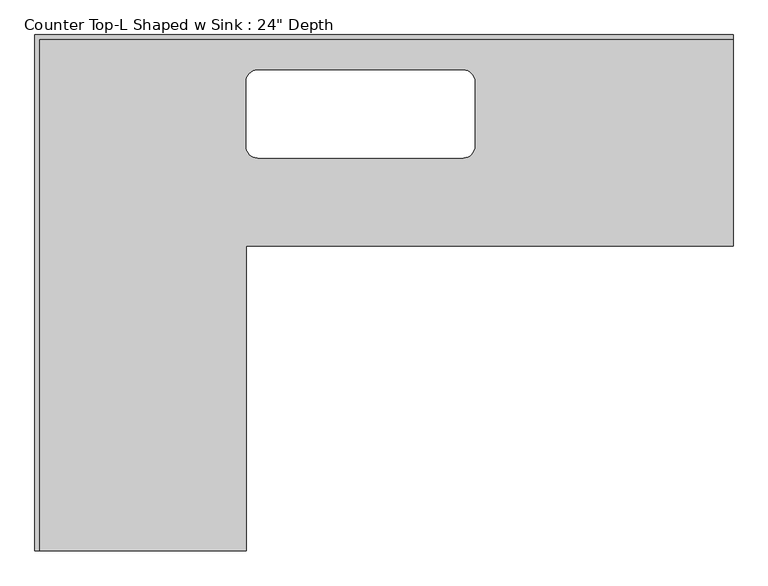
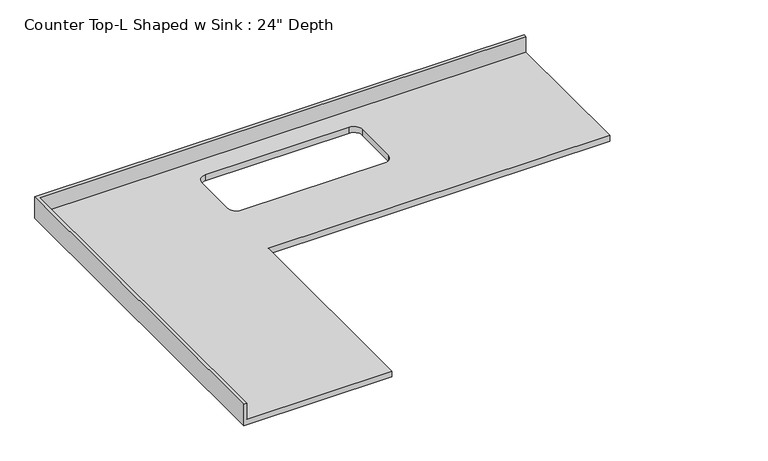
"""IFC4 building model written with IfcOpenShell, lengths in millimetres: furniture geometry."""

from ifc_helpers import new_model, si_unit, frame, origin, place, context, project, spatial, polyline, circle_curve, source, transform, mapped, element, save
from ifc_brep_helpers import plane_surface, revolved_surface, advanced_brep


def furniture_51338070(model_context):
    return source(origin(), model_context, "Body", "AdvancedBrep", [
        advanced_brep(
        [(-286.0622951, -2236.5215516, 914.4), (-286.0622951, -914.4, 914.4), (1823.297737, -914.4, 914.4), (1823.297737, -19.05, 914.4), (-1181.4122951, -19.05, 914.4), (-1181.4122951, -2236.5215516, 914.4), (653.7377049, -152.4, 914.4), (704.5377049, -203.2, 914.4), (704.5377049, -482.6, 914.4), (653.7377049, -533.4, 914.4), (-235.2622951, -533.4, 914.4), (-286.0622951, -482.6, 914.4), (-286.0622951, -203.2, 914.4), (-235.2622951, -152.4, 914.4), (1823.297737, 0.0, 876.3), (1823.297737, -914.4, 876.3), (-286.0622951, -914.4, 876.3), (-286.0622951, -2236.5215516, 876.3), (-1200.4622951, -2236.5215516, 876.3), (-1200.4622951, 0.0, 876.3), (653.7377049, -152.4, 876.3), (-235.2622951, -152.4, 876.3), (-286.0622951, -203.2, 876.3), (-286.0622951, -482.6, 876.3), (-235.2622951, -533.4, 876.3), (653.7377049, -533.4, 876.3), (704.5377049, -482.6, 876.3), (704.5377049, -203.2, 876.3), (-1200.4622951, 0.0, 1016.0), (1823.297737, 0.0, 1016.0), (-1200.4622951, -2236.5215516, 1016.0), (-1181.4122951, -2236.5215516, 1016.0), (1823.297737, -19.05, 1016.0), (-1181.4122951, -19.05, 1016.0)],
        [
            (0, 1),
            (1, 2),
            (2, 3),
            (3, 4),
            (4, 5),
            (5, 0),
            (6, 7, circle_curve(frame((653.7377049, -203.2, 914.4), z_axis=(0.0, 0.0, -1.0), x_axis=(1.0, 0.0, 0.0)), 50.8)),
            (7, 8),
            (8, 9, circle_curve(frame((653.7377049, -482.6, 914.4), z_axis=(0.0, 0.0, -1.0), x_axis=(1.0, 0.0, 0.0)), 50.8)),
            (9, 10),
            (10, 11, circle_curve(frame((-235.2622951, -482.6, 914.4), z_axis=(0.0, 0.0, -1.0), x_axis=(1.0, 0.0, 0.0)), 50.8)),
            (11, 12),
            (12, 13, circle_curve(frame((-235.2622951, -203.2, 914.4), z_axis=(0.0, 0.0, -1.0), x_axis=(1.0, 0.0, 0.0)), 50.8)),
            (13, 6),
            (14, 15),
            (15, 16),
            (16, 17),
            (17, 18),
            (18, 19),
            (19, 14),
            (20, 21),
            (21, 22, circle_curve(frame((-235.2622951, -203.2, 876.3), z_axis=(0.0, 0.0, 1.0), x_axis=(1.0, 0.0, 0.0)), 50.8)),
            (22, 23),
            (23, 24, circle_curve(frame((-235.2622951, -482.6, 876.3), z_axis=(0.0, 0.0, 1.0), x_axis=(1.0, 0.0, 0.0)), 50.8)),
            (24, 25),
            (25, 26, circle_curve(frame((653.7377049, -482.6, 876.3), z_axis=(0.0, 0.0, 1.0), x_axis=(1.0, 0.0, 0.0)), 50.8)),
            (26, 27),
            (27, 20, circle_curve(frame((653.7377049, -203.2, 876.3), z_axis=(0.0, 0.0, 1.0), x_axis=(1.0, 0.0, 0.0)), 50.8)),
            (19, 28),
            (28, 29),
            (29, 14),
            (18, 30),
            (30, 28),
            (17, 0),
            (5, 31),
            (31, 30),
            (16, 1),
            (15, 2),
            (29, 32),
            (32, 3),
            (6, 20),
            (27, 7),
            (26, 8),
            (25, 9),
            (24, 10),
            (23, 11),
            (22, 12),
            (21, 13),
            (31, 33),
            (33, 32),
            (33, 4),
        ],
        [
            plane_surface(frame((-1200.4622951, 0.0, 914.4), z_axis=(0.0, 0.0, 1.0), x_axis=(-1.0, 0.0, 0.0))),
            plane_surface(frame((-1200.4622951, 0.0, 876.3), z_axis=(0.0, 0.0, -1.0), x_axis=(1.0, 0.0, 0.0))),
            plane_surface(frame((1823.297737, 0.0, 914.4), z_axis=(0.0, 1.0, 0.0), x_axis=(0.0, 0.0, -1.0))),
            plane_surface(frame((-1200.4622951, 0.0, 914.4), z_axis=(-1.0, 0.0, 0.0), x_axis=(0.0, 0.0, -1.0))),
            plane_surface(frame((-1200.4622951, -2236.5215516, 914.4), z_axis=(0.0, -1.0, 0.0), x_axis=(0.0, 0.0, -1.0))),
            plane_surface(frame((-286.0622951, -2236.5215516, 914.4), z_axis=(1.0, 0.0, 0.0), x_axis=(0.0, 0.0, -1.0))),
            plane_surface(frame((-286.0622951, -914.4, 914.4), z_axis=(0.0, -1.0, 0.0), x_axis=(0.0, 0.0, -1.0))),
            plane_surface(frame((1823.297737, -914.4, 914.4), z_axis=(1.0, 0.0, 0.0), x_axis=(0.0, 0.0, -1.0))),
            revolved_surface(polyline([(704.5377049, -203.2, 876.3), (704.5377049, -203.2, 914.4)]), (653.7377049, -203.2, 0.0), (0.0, 0.0, -1.0)),
            plane_surface(frame((704.5377049, -203.2, 914.4), z_axis=(-1.0, 0.0, 0.0), x_axis=(0.0, 0.0, -1.0))),
            revolved_surface(polyline([(704.5377049, -482.6, 876.3), (704.5377049, -482.6, 914.4)]), (653.7377049, -482.6, 0.0), (0.0, 0.0, -1.0)),
            plane_surface(frame((653.7377049, -533.4, 914.4), z_axis=(0.0, 1.0, 0.0), x_axis=(0.0, 0.0, -1.0))),
            revolved_surface(polyline([(-184.4622951, -482.6, 876.3), (-184.4622951, -482.6, 914.4)]), (-235.2622951, -482.6, 0.0), (0.0, 0.0, -1.0)),
            plane_surface(frame((-286.0622951, -482.6, 914.4), z_axis=(1.0, 0.0, 0.0), x_axis=(0.0, 0.0, -1.0))),
            revolved_surface(polyline([(-184.4622951, -203.2, 876.3), (-184.4622951, -203.2, 914.4)]), (-235.2622951, -203.2, 0.0), (0.0, 0.0, -1.0)),
            plane_surface(frame((-235.2622951, -152.4, 914.4), z_axis=(0.0, -1.0, 0.0), x_axis=(0.0, 0.0, -1.0))),
            plane_surface(frame((-1200.4622951, 0.0, 1016.0), z_axis=(0.0, 0.0, 1.0), x_axis=(0.0, -1.0, 0.0))),
            plane_surface(frame((-1200.4622951, -19.05, 1016.0), z_axis=(0.0, -1.0, 0.0), x_axis=(0.0, 0.0, -1.0))),
            plane_surface(frame((-1181.4122951, -2236.5215516, 1016.0), z_axis=(1.0, 0.0, 0.0), x_axis=(0.0, 0.0, -1.0))),
        ],
        [
            (0, [[1, 2, 3, 4, 5, 6], [7, 8, 9, 10, 11, 12, 13, 14]]),
            (1, [[15, 16, 17, 18, 19, 20], [21, 22, 23, 24, 25, 26, 27, 28]]),
            (2, [[-20, 29, 30, 31]]),
            (3, [[-19, 32, 33, -29]]),
            (4, [[-32, -18, 34, -6, 35, 36]]),
            (5, [[-1, -34, -17, 37]]),
            (6, [[-2, -37, -16, 38]]),
            (7, [[-15, -31, 39, 40, -3, -38]]),
            (8, [[-7, 41, -28, 42]]),
            (9, [[-8, -42, -27, 43]]),
            (10, [[-9, -43, -26, 44]]),
            (11, [[-10, -44, -25, 45]]),
            (12, [[-11, -45, -24, 46]]),
            (13, [[-12, -46, -23, 47]]),
            (14, [[-13, -47, -22, 48]]),
            (15, [[-14, -48, -21, -41]]),
            (16, [[-33, -36, 49, 50, -39, -30]]),
            (17, [[-40, -50, 51, -4]]),
            (18, [[-49, -35, -5, -51]]),
        ],
    ),
    ])


if __name__ == "__main__":
    model = new_model("IFC4")
    model_context = context("Model", 3, world=origin())
    ifc_project = project(units=[si_unit("LENGTHUNIT", "METRE", prefix="MILLI")], contexts=[model_context])
    site = spatial("IfcSite", under=ifc_project)
    building = spatial("IfcBuilding", under=site)
    placement = place(None, origin())
    furniture_shape = furniture_51338070(model_context)
    element("IfcFurniture", 1, ObjectType="Counter Top-L Shaped w Sink : 24\" Depth", at=placement, inside=building, context=model_context, shape_type="MappedRepresentation", body=[
        mapped(furniture_shape, transform((0.0, 0.0, 0.0), x_axis=(1.0, 0.0, 0.0), y_axis=(0.0, 1.0, 0.0), z_axis=(0.0, 0.0, 1.0))),
    ])
    save(model, "model.ifc")

# Revit data of these elements
# Type "Counter Top-L Shaped w Sink : 24\" Depth"
#   Assembly Code = "C1030400"
#   Counter Thickness = 0' - 1 1/2"
#   Depth = 3' - 0"
#   Height = 3' - 0"
#   Length - Leg 1 [instance default] = 8' - 0"
#   Length - Leg 2 [instance default] = 6' - 0"
#   Sink Location [instance default] = 3' - 0"
#   Sink Location To Wall [instance default] = 0' - 6"
#   Sink Opening Depth [instance default] = 1' - 3"
#   Sink Opening Width [instance default] = 3' - 3"
#   Counter Top Material = none
#   Default Elevation = 0
# Element 1 (IfcFurniture, "Counter Top-L Shaped w Sink : 24\" Depth")
#   Length - Leg 1 = 9' - 11.04567"
#   Length - Leg 2 = 7' - 4.05203"
#   Materials on its faces: "Counter Top"
# Materials
#   "Counter Top": class "Wood", colour RGB 226 177 128, transparency 0
